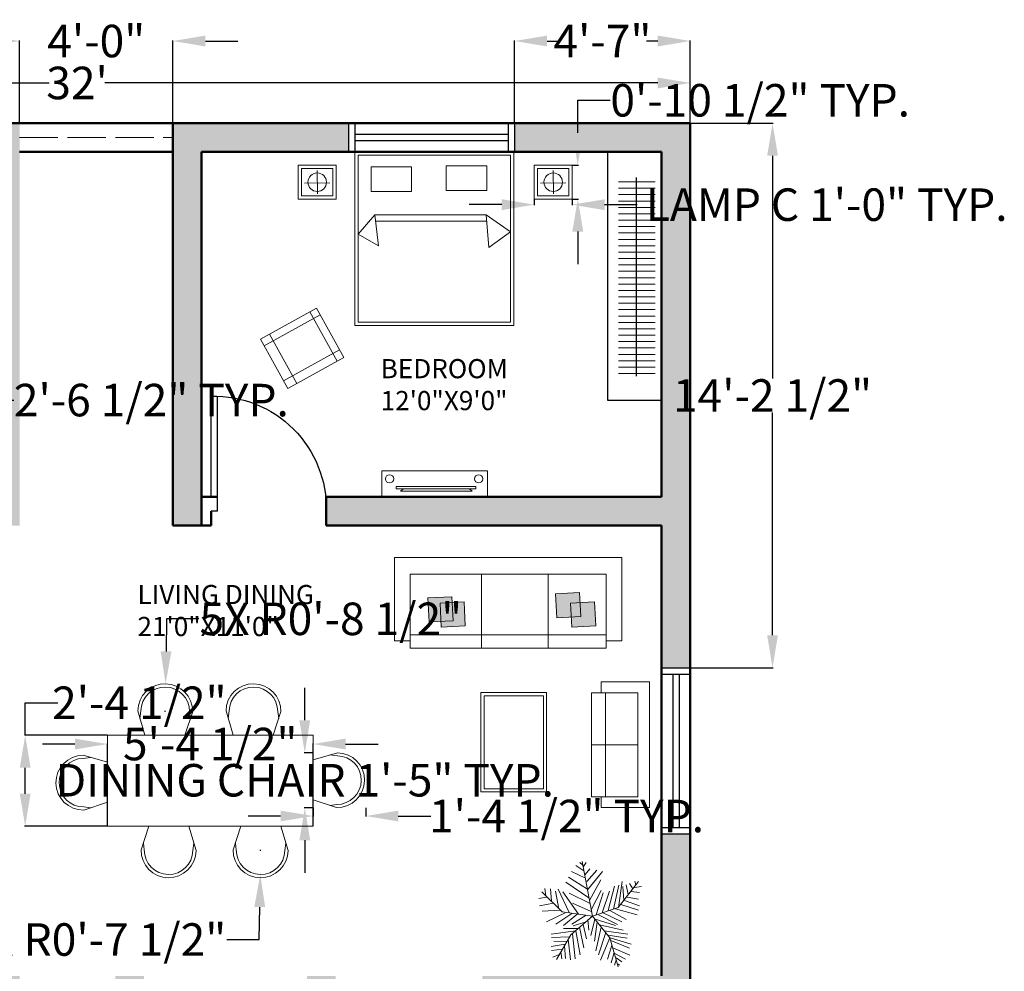
# Model space of a CAD drawing. Units: inches. Extents: x 18 to 9768, y 4 to 3529.
# Tile 6 of 6: x 9424 to 9733, y 3225 to 3523. Entities that reach past the tile are written whole.
import ezdxf

# ---------------------------------------------------------------- set-up
doc = ezdxf.new("R2010")
doc.units = ezdxf.units.IN
doc.header["$MEASUREMENT"] = 0
doc.linetypes.add('ACAD_ISO02W100', pattern=[15, 12, -3])
for name, color, linetype, lineweight in [('A-ANNO-DIMS', 2, 'Continuous', 18), ('A-AREA-IDEN', 7, 'Continuous', 18), ('A-CASE-PATT', 9, 'Continuous', 13), ('A-EQPM', 8, 'Continuous', 18), ('A-FLOR-CASE', 9, 'Continuous', 25), ('A-FURN', 8, 'Continuous', 18), ('A-FURN-PATT', 9, 'Continuous', 13), ('A-WALL-OVHD', 8, 'ACAD_ISO02W100', 18), ('A-WALL-PATT', 252, 'Continuous', 13), ('L-PLNT', 3, 'Continuous', 18), ('WAL', 7, 'Continuous', 50)]:
    doc.layers.add(name, color=color, linetype=linetype, lineweight=lineweight)
doc.layers.add('A-DOOR', color=30, linetype='Continuous', lineweight=25, true_color=0xf8991e)
doc.layers.add('A-GLAZ', color=177, linetype='Continuous', lineweight=25, true_color=0x293189)
doc.styles.get("Standard").update_dxf_attribs({"font": 'arial.ttf'})
doc.dimstyles.get("Standard").update_dxf_attribs({"dimtxt": 10.18, "dimasz": 10.18, "dimexe": 0.18, "dimexo": 0.0625, "dimgap": 0.09, "dimtad": 0, "dimtih": 1, "dimtoh": 1, "dimdec": 0, "dimzin": 0, "dimdsep": 46, "dimlunit": 3, "dimtxsty": 'Standard', "dimcen": 0.09, "dimadec": 0, "dimazin": 0, "dimtfac": 1, "dimtdec": 0, "dimtofl": 0, "dimtmove": 0, "dimatfit": 3, "dimfxl": 1, "dimtolj": 1, "dimtzin": 0, "dimarcsym": 0})

# ---------------------------------------------------------------- blocks, each defined once
blk = doc.blocks.new('*U6')
for p, q in [((-8.737, 47.138), (-17.069, 52.711)), ((-10.186, 53.64), (-13.084, 55.962)), ((0, 0), (-10.5, 57)), ((-9.099, 51.782), (-6.563, 55.962)), ((-7.288, 39.707), (-21.778, 46.673)), ((-7.65, 43.423), (-2.578, 49.46)), ((-5.839, 35.992), (4.667, 48.067)), ((-5.114, 27.632), (10.463, 46.673)), ((-3.665, 19.273), (-27.574, 35.527)), ((-5.114, 28.097), (-24.676, 40.636)), ((-2.941, 16.486), (8.652, 37.85)), ((16.259, 5.805), (23.142, 31.348)), ((22.055, 7.198), (27.489, 32.277)), ((27, 9), (48, 36)), ((27.127, 9.056), (31.112, 35.992)), ((31.836, 30.883), (32.561, 16.486)), ((35.096, 32.741), (37.27, 22.524)), ((38.719, 34.134), (41.979, 28.561)), ((43.791, 29.954), (51.036, 30.883)), ((44.153, 36.456), (45.239, 32.741)), ((-31.5, 4.5), (-52.5, 25.5)), ((-48.585, 21.131), (-49.309, 29.026)), ((-43.513, 28.561), (-42.427, 15.558)), ((-38.442, 26.239), (-34.819, 7.663)), ((-35.544, 28.097), (-24.314, 3.947)), ((-14.533, 2.09), (-30.834, 25.31)), ((-24.314, 23.917), (-2.941, 13.7)), ((-1.129, 6.734), (9.014, 26.704)), ((3.942, 1.625), (11.187, 24.381)), ((10.101, 3.483), (17.708, 26.239)), ((40.53, 25.775), (48.862, 24.846)), ((-47.498, 19.737), (-55.83, 18.344)), ((-40.615, 13.7), (-55.105, 10.913)), ((-20.691, 13.7), (-1.129, 4.876)), ((29.662, 12.307), (48.137, 6.269)), ((33.285, 16.486), (48.862, 10.913)), ((36.183, 19.737), (48.137, 17.88)), ((-33.37, 6.269), (-52.207, 5.34)), ((-28.299, 3.483), (-47.86, -5.805)), ((-21.416, 3.018), (-38.079, -8.128)), ((0, 0), (-31.5, 4.5)), ((-15.982, 2.09), (-30.11, -9.521)), ((0, 0), (-22.5, -19.5)), ((-6.563, 1.161), (-21.416, -8.128)), ((0, 0), (27, 9)), ((0, 0), (18, -22.5)), ((6.478, 1.625), (26.04, -8.592)), ((11.187, 3.483), (30.749, -5.805)), ((18.07, 5.805), (35.096, -3.483)), ((24.229, 7.663), (46.688, 1.625)), ((-6.563, -5.805), (-19.967, -9.985)), ((-9.461, -8.592), (-6.201, -23.453)), ((-4.752, -3.483), (-3.665, -14.629)), ((2.493, -3.019), (-1.491, -20.202)), ((1.769, -2.555), (24.229, -9.521)), ((5.029, -6.27), (2.131, -25.775)), ((7.565, -9.056), (32.198, -14.629)), ((-17.431, -15.094), (-42.789, -18.809)), ((-22.5, -19.5), (-37.5, -45)), ((-15.257, -12.772), (-30.11, -12.772)), ((-20.691, -18.345), (-17.793, -44.352)), ((-17.069, -15.094), (-12.721, -40.172)), ((-13.446, -11.378), (-8.737, -32.741)), ((9.014, -11.378), (3.58, -35.992)), ((14.085, -16.951), (6.478, -40.172)), ((12.274, -15.094), (36.907, -18.809)), ((16.259, -19.738), (36.183, -22.989)), ((-28.299, -29.026), (-42.789, -31.348)), ((-24.314, -21.596), (-42.427, -22.06)), ((-26.849, -26.24), (-40.253, -25.775)), ((-25.038, -23.918), (-22.865, -45.281)), ((18.07, -22.524), (8.289, -45.745)), ((20.244, -30.419), (15.897, -44.816)), ((18, -22.5), (27, -52.5)), ((18.433, -22.524), (40.53, -29.026)), ((19.157, -25.311), (38.719, -33.206)), ((-30.834, -34.135), (-42.427, -35.528)), ((-34.457, -39.708), (-40.978, -42.494)), ((-32.646, -36.921), (-31.921, -44.352)), ((-29.023, -30.884), (-27.936, -43.887)), ((22.78, -37.85), (19.519, -48.532)), ((21.331, -32.741), (39.081, -40.636)), ((22.78, -38.314), (34.372, -44.816)), ((24.591, -45.745), (23.142, -50.854)), ((24.591, -43.423), (30.749, -47.603)), ((26.764, -49.925), (28.213, -50.854))]:
    blk.add_line(p, q)
blk = doc.blocks.new('*D7')
at = {"layer": 'A-ANNO-DIMS', "color": 0, "lineweight": -2, "transparency": 16777216}
for p, q in [((9250.43, 3490.42), (9250.43, 3503.16)), ((9260.61, 3502.98), (9433.71, 3502.98)), ((9624.25, 3502.98), (9451.16, 3502.98)), ((9634.43, 3490.42), (9634.43, 3503.16))]:
    blk.add_line(p, q, dxfattribs=at)
at = {"layer": 'A-ANNO-DIMS', "color": 0, "transparency": 16777216}
for points in [[(9260.61, 3504.67), (9260.61, 3501.28), (9250.43, 3502.98)], [(9624.25, 3504.67), (9624.25, 3501.28), (9634.43, 3502.98)]]:
    blk.add_solid(points, dxfattribs=at)
at = {"layer": 'Defpoints', "color": 0, "transparency": 16777216}
for p in [(9634.43, 3502.98), (9250.43, 3490.36), (9634.43, 3490.36)]:
    blk.add_point(p, dxfattribs=at)
at = {"layer": 'A-ANNO-DIMS', "color": 0, "transparency": 16777216, "insert": (9442.43, 3502.98), "char_height": 10.18, "attachment_point": 5}
blk.add_mtext("\\A1;32'", dxfattribs=at)
blk = doc.blocks.new('WINDOW-48')
for p, q in [((0, 0), (0, 9)), ((2, 0), (2, 9)), ((50, 0), (50, 9)), ((52, 0), (52, 9)), ((2, 5.5), (50, 5.5)), ((2, 3.5), (50, 3.5))]:
    blk.add_line(p, q)
blk = doc.blocks.new('DOOR-36-W9')
for p, q in [((2, 36.01), (0, 36.01)), ((2, 36.01), (2, 0.01)), ((0, 31.51), (0, 0.01))]:
    blk.add_line(p, q)
blk.add_arc((1, 35.01), 35.01, 268.3634, 1.6366)
blk = doc.blocks.new('CHAIR-DINING')
for p, q in [((0, 7.62), (2.22, 0)), ((1, 7.61), (0.68, 5.29)), ((14.73, 0), (17.19, 7.39)), ((16.19, 7.4), (16.49, 5.29))]:
    blk.add_line(p, q)
for radius in [8.6, 7.6]:
    blk.add_arc((8.59, 7.51), radius, 359.2162, 179.2162)
blk = doc.blocks.new('NIGHTSTAND-LAMP-C')
for p, q in [((5.92, 8.89), (5.98, 1.61)), ((1.92, 5.01), (9.92, 5.04))]:
    blk.add_line(p, q)
for points in [[(0, 10.55), (0, 10.55), (11.83, 10.55), (11.83, 10.55), (11.83, 0), (11.83, 0), (0, 0), (0, 0)], [(1, 9.55), (10.83, 9.55), (10.83, 1), (1, 1)]]:
    blk.add_lwpolyline(points, close=True)
blk.add_circle((5.92, 5.27), 2.89)
blk = doc.blocks.new('*D36')
at = {"layer": 'A-ANNO-DIMS', "color": 0, "lineweight": -2, "transparency": 16777216}
for p, q in [((9382.16, 3399.2), (9382.16, 3403.86)), ((9392.34, 3403.68), (9402.25, 3403.68)), ((9412.43, 3399.2), (9412.43, 3403.86)), ((9412.43, 3403.68), (9422.61, 3403.68))]:
    blk.add_line(p, q, dxfattribs=at)
at = {"layer": 'A-ANNO-DIMS', "color": 0, "transparency": 16777216}
for points in [[(9392.34, 3405.38), (9392.34, 3401.98), (9382.16, 3403.68)], [(9402.25, 3405.38), (9402.25, 3401.98), (9412.43, 3403.68)]]:
    blk.add_solid(points, dxfattribs=at)
at = {"layer": 'Defpoints', "color": 0, "transparency": 16777216}
for p in [(9412.43, 3403.68), (9382.16, 3399.14), (9412.43, 3399.14)]:
    blk.add_point(p, dxfattribs=at)
at = {"layer": 'A-ANNO-DIMS', "color": 0, "transparency": 16777216, "insert": (9465.68, 3403.68), "char_height": 10.18, "attachment_point": 5}
blk.add_mtext('\\A1;2\'-6 1/2" TYP.', dxfattribs=at)
blk = doc.blocks.new('*D37')
at = {"layer": 'A-ANNO-DIMS', "color": 0, "lineweight": -2, "transparency": 16777216}
for p, q in [((9513.73, 3303.43), (9513.73, 3313.61)), ((9516.25, 3293.25), (9513.55, 3293.25)), ((9516.25, 3276.02), (9513.55, 3276.02)), ((9513.73, 3265.84), (9513.73, 3255.66))]:
    blk.add_line(p, q, dxfattribs=at)
at = {"layer": 'A-ANNO-DIMS', "color": 0, "transparency": 16777216}
for points in [[(9512.03, 3303.43), (9515.42, 3303.43), (9513.73, 3293.25)], [(9512.03, 3265.84), (9515.42, 3265.84), (9513.73, 3276.02)]]:
    blk.add_solid(points, dxfattribs=at)
at = {"layer": 'Defpoints', "color": 0, "transparency": 16777216}
for p in [(9516.31, 3293.25), (9513.73, 3276.02), (9516.31, 3276.02)]:
    blk.add_point(p, dxfattribs=at)
at = {"layer": 'A-ANNO-DIMS', "color": 0, "transparency": 16777216, "insert": (9513.73, 3284.63), "char_height": 10.18, "attachment_point": 5}
blk.add_mtext('\\A1;DINING CHAIR 1\'-5" TYP.', dxfattribs=at)
blk = doc.blocks.new('*D38')
at = {"layer": 'A-ANNO-DIMS', "color": 0, "lineweight": -2, "transparency": 16777216}
for p, q in [((9516.31, 3275.95), (9516.31, 3273.25)), ((9532.82, 3275.95), (9532.82, 3273.25)), ((9506.13, 3273.43), (9495.95, 3273.43)), ((9543, 3273.43), (9553.18, 3273.43))]:
    blk.add_line(p, q, dxfattribs=at)
at = {"layer": 'A-ANNO-DIMS', "color": 0, "transparency": 16777216}
for points in [[(9506.13, 3275.13), (9506.13, 3271.74), (9516.31, 3273.43)], [(9543, 3275.13), (9543, 3271.74), (9532.82, 3273.43)]]:
    blk.add_solid(points, dxfattribs=at)
at = {"layer": 'Defpoints', "color": 0, "transparency": 16777216}
for p in [(9516.31, 3276.02), (9532.82, 3276.02), (9532.82, 3273.43)]:
    blk.add_point(p, dxfattribs=at)
at = {"layer": 'A-ANNO-DIMS', "color": 0, "transparency": 16777216, "insert": (9595.68, 3273.43), "char_height": 10.18, "attachment_point": 5}
blk.add_mtext('\\A1;1\'-4 1/2" TYP.', dxfattribs=at)
blk = doc.blocks.new('*D51')
at = {"layer": 'A-ANNO-DIMS', "color": 0, "lineweight": -2, "transparency": 16777216}
for p, q in [((9585.59, 3466.58), (9585.59, 3464.69)), ((9597.43, 3466.58), (9597.43, 3464.69)), ((9575.41, 3464.87), (9565.23, 3464.87)), ((9607.61, 3464.87), (9617.79, 3464.87))]:
    blk.add_line(p, q, dxfattribs=at)
at = {"layer": 'A-ANNO-DIMS', "color": 0, "transparency": 16777216}
for points in [[(9575.41, 3466.56), (9575.41, 3463.17), (9585.59, 3464.87)], [(9607.61, 3466.56), (9607.61, 3463.17), (9597.43, 3464.87)]]:
    blk.add_solid(points, dxfattribs=at)
at = {"layer": 'Defpoints', "color": 0, "transparency": 16777216}
for p in [(9585.59, 3466.64), (9597.43, 3466.64), (9597.43, 3464.87)]:
    blk.add_point(p, dxfattribs=at)
at = {"layer": 'A-ANNO-DIMS', "color": 0, "transparency": 16777216, "insert": (9677.13, 3464.87), "char_height": 10.18, "attachment_point": 5}
blk.add_mtext('\\A1;LAMP C 1\'-0" TYP.', dxfattribs=at)
blk = doc.blocks.new('*D52')
at = {"layer": 'A-ANNO-DIMS', "color": 0, "lineweight": -2, "transparency": 16777216}
for p, q in [((9599.2, 3487.37), (9599.2, 3497.55)), ((9599.2, 3497.55), (9609.38, 3497.55)), ((9597.49, 3477.19), (9599.38, 3477.19)), ((9597.49, 3466.64), (9599.38, 3466.64)), ((9599.2, 3456.46), (9599.2, 3446.28))]:
    blk.add_line(p, q, dxfattribs=at)
at = {"layer": 'A-ANNO-DIMS', "color": 0, "transparency": 16777216}
for points in [[(9597.51, 3487.37), (9600.9, 3487.37), (9599.2, 3477.19)], [(9597.51, 3456.46), (9600.9, 3456.46), (9599.2, 3466.64)]]:
    blk.add_solid(points, dxfattribs=at)
at = {"layer": 'Defpoints', "color": 0, "transparency": 16777216}
for p in [(9597.43, 3477.19), (9599.2, 3477.19), (9597.43, 3466.64)]:
    blk.add_point(p, dxfattribs=at)
at = {"layer": 'A-ANNO-DIMS', "color": 0, "transparency": 16777216, "insert": (9656.31, 3497.55), "char_height": 10.18, "attachment_point": 5}
blk.add_mtext('\\A1;0\'-10 1/2" TYP.', dxfattribs=at)
blk = doc.blocks.new('*D72')
at = {"layer": 'A-ANNO-DIMS', "color": 0, "lineweight": -2, "transparency": 16777216}
for p, q in [((9414.25, 3516.11), (9404.07, 3516.11)), ((9424.43, 3490.42), (9424.43, 3516.29)), ((9472.43, 3490.42), (9472.43, 3516.29)), ((9482.61, 3516.11), (9492.79, 3516.11))]:
    blk.add_line(p, q, dxfattribs=at)
at = {"layer": 'A-ANNO-DIMS', "color": 0, "transparency": 16777216}
for points in [[(9414.25, 3517.81), (9414.25, 3514.41), (9424.43, 3516.11)], [(9482.61, 3517.81), (9482.61, 3514.41), (9472.43, 3516.11)]]:
    blk.add_solid(points, dxfattribs=at)
at = {"layer": 'Defpoints', "color": 0, "transparency": 16777216}
for p in [(9472.43, 3516.11), (9424.43, 3490.36), (9472.43, 3490.36)]:
    blk.add_point(p, dxfattribs=at)
at = {"layer": 'A-ANNO-DIMS', "color": 0, "transparency": 16777216, "insert": (9448.43, 3516.11), "char_height": 10.18, "attachment_point": 5}
blk.add_mtext('\\A1;4\'-0"', dxfattribs=at)
blk = doc.blocks.new('*D74')
at = {"layer": 'A-ANNO-DIMS', "color": 0, "lineweight": -2, "transparency": 16777216}
for p, q in [((9579.43, 3490.42), (9579.43, 3516.29)), ((9589.61, 3516.11), (9593.11, 3516.11)), ((9624.25, 3516.11), (9620.76, 3516.11)), ((9634.43, 3490.42), (9634.43, 3516.29))]:
    blk.add_line(p, q, dxfattribs=at)
at = {"layer": 'A-ANNO-DIMS', "color": 0, "transparency": 16777216}
for points in [[(9589.61, 3517.81), (9589.61, 3514.41), (9579.43, 3516.11)], [(9624.25, 3517.81), (9624.25, 3514.41), (9634.43, 3516.11)]]:
    blk.add_solid(points, dxfattribs=at)
at = {"layer": 'Defpoints', "color": 0, "transparency": 16777216}
for p in [(9634.43, 3516.11), (9579.43, 3490.36), (9634.43, 3490.36)]:
    blk.add_point(p, dxfattribs=at)
at = {"layer": 'A-ANNO-DIMS', "color": 0, "transparency": 16777216, "insert": (9606.93, 3516.11), "char_height": 10.18, "attachment_point": 5}
blk.add_mtext('\\A1;4\'-7"', dxfattribs=at)
blk = doc.blocks.new('*D77')
at = {"layer": 'A-ANNO-DIMS', "color": 0, "lineweight": -2, "transparency": 16777216}
for p, q in [((9634.5, 3490.36), (9660.36, 3490.36)), ((9660.18, 3480.18), (9660.18, 3410.46)), ((9660.18, 3330.04), (9660.18, 3399.76)), ((9634.5, 3319.86), (9660.36, 3319.86))]:
    blk.add_line(p, q, dxfattribs=at)
at = {"layer": 'A-ANNO-DIMS', "color": 0, "transparency": 16777216}
for points in [[(9658.49, 3480.18), (9661.88, 3480.18), (9660.18, 3490.36)], [(9658.49, 3330.04), (9661.88, 3330.04), (9660.18, 3319.86)]]:
    blk.add_solid(points, dxfattribs=at)
at = {"layer": 'Defpoints', "color": 0, "transparency": 16777216}
for p in [(9634.43, 3490.36), (9660.18, 3490.36), (9634.43, 3319.86)]:
    blk.add_point(p, dxfattribs=at)
at = {"layer": 'A-ANNO-DIMS', "color": 0, "transparency": 16777216, "insert": (9660.18, 3405.11), "char_height": 10.18, "attachment_point": 5}
blk.add_mtext('\\A1;14\'-2 1/2"', dxfattribs=at)
blk = doc.blocks.new('*D79')
at = {"layer": 'A-ANNO-DIMS', "color": 0, "lineweight": -2, "transparency": 16777216}
for p, q in [((9441.75, 3295.97), (9431.57, 3295.97)), ((9451.93, 3270.28), (9451.93, 3296.15)), ((9516.31, 3270.28), (9516.31, 3296.15)), ((9526.49, 3295.97), (9536.67, 3295.97))]:
    blk.add_line(p, q, dxfattribs=at)
at = {"layer": 'A-ANNO-DIMS', "color": 0, "transparency": 16777216}
for points in [[(9441.75, 3297.66), (9441.75, 3294.27), (9451.93, 3295.97)], [(9526.49, 3297.66), (9526.49, 3294.27), (9516.31, 3295.97)]]:
    blk.add_solid(points, dxfattribs=at)
at = {"layer": 'Defpoints', "color": 0, "transparency": 16777216}
for p in [(9516.31, 3295.97), (9451.93, 3270.22), (9516.31, 3270.22)]:
    blk.add_point(p, dxfattribs=at)
at = {"layer": 'A-ANNO-DIMS', "color": 0, "transparency": 16777216, "insert": (9484.12, 3295.97), "char_height": 10.18, "attachment_point": 5}
blk.add_mtext('\\A1;5\'-4 1/2"', dxfattribs=at)
blk = doc.blocks.new('*D80')
at = {"layer": 'A-ANNO-DIMS', "color": 0, "lineweight": -2, "transparency": 16777216}
for p, q in [((9426.18, 3298.72), (9426.18, 3308.9)), ((9426.18, 3308.9), (9436.36, 3308.9)), ((9451.87, 3298.72), (9426, 3298.72)), ((9426.18, 3280.4), (9426.18, 3288.54)), ((9451.87, 3270.22), (9426, 3270.22))]:
    blk.add_line(p, q, dxfattribs=at)
at = {"layer": 'A-ANNO-DIMS', "color": 0, "transparency": 16777216}
for points in [[(9424.48, 3288.54), (9427.88, 3288.54), (9426.18, 3298.72)], [(9424.48, 3280.4), (9427.88, 3280.4), (9426.18, 3270.22)]]:
    blk.add_solid(points, dxfattribs=at)
at = {"layer": 'Defpoints', "color": 0, "transparency": 16777216}
for p in [(9426.18, 3298.72), (9451.93, 3298.72), (9451.93, 3270.22)]:
    blk.add_point(p, dxfattribs=at)
at = {"layer": 'A-ANNO-DIMS', "color": 0, "transparency": 16777216, "insert": (9461.93, 3308.9), "char_height": 10.18, "attachment_point": 5}
blk.add_mtext('\\A1;2\'-4 1/2"', dxfattribs=at)
blk = doc.blocks.new('*D83')
at = {"layer": 'A-ANNO-DIMS', "color": 0, "lineweight": -2, "transparency": 16777216}
for p, q in [((9470.42, 3335.18), (9470.28, 3325)), ((9480.6, 3335.18), (9470.42, 3335.18)), ((9469.93, 3306.23), (9470.11, 3306.23)), ((9470.02, 3306.14), (9470.02, 3306.32))]:
    blk.add_line(p, q, dxfattribs=at)
at = {"layer": 'A-ANNO-DIMS', "color": 0, "transparency": 16777216}
blk.add_solid([(9468.58, 3325.03), (9471.97, 3324.98), (9470.14, 3314.82)], dxfattribs=at)
at = {"layer": 'Defpoints', "color": 0, "transparency": 16777216}
for p in [(9470.14, 3314.82), (9470.02, 3306.23)]:
    blk.add_point(p, dxfattribs=at)
at = {"layer": 'A-ANNO-DIMS', "color": 0, "transparency": 16777216, "insert": (9521.89, 3335.18), "char_height": 10.18, "attachment_point": 5}
blk.add_mtext('\\A1;5X R0\'-8 1/2"', dxfattribs=at)
blk = doc.blocks.new('*D84')
at = {"layer": 'A-ANNO-DIMS', "color": 0, "lineweight": -2, "transparency": 16777216}
for p, q in [((9499.78, 3262.71), (9499.96, 3262.71)), ((9499.87, 3262.62), (9499.87, 3262.8)), ((9499.49, 3234.76), (9499.63, 3244.93)), ((9489.31, 3234.76), (9499.49, 3234.76))]:
    blk.add_line(p, q, dxfattribs=at)
at = {"layer": 'A-ANNO-DIMS', "color": 0, "transparency": 16777216}
blk.add_solid([(9497.93, 3244.96), (9501.32, 3244.91), (9499.77, 3255.11)], dxfattribs=at)
at = {"layer": 'Defpoints', "color": 0, "transparency": 16777216}
for p in [(9499.87, 3262.71), (9499.77, 3255.11)]:
    blk.add_point(p, dxfattribs=at)
at = {"layer": 'A-ANNO-DIMS', "color": 0, "transparency": 16777216, "insert": (9448.02, 3234.76), "char_height": 10.18, "attachment_point": 5}
blk.add_mtext('\\A1;5X R0\'-7 1/2"', dxfattribs=at)

msp = doc.modelspace()

# ---------------------------------------------------------------- hatches: boundary and pattern name
at = {"layer": 'A-CASE-PATT'}
h = msp.add_hatch(dxfattribs=at)
h.set_pattern_fill('ANSI31', color=256, scale=16, angle=-45, style=0)
h.paths.add_polyline_path([(9612, 3410.74), (9623.39, 3410.74), (9623.39, 3472.74), (9612, 3472.74)])
at = {"layer": 'A-FURN-PATT'}
h = msp.add_hatch(color=256, dxfattribs=at)
h.dxf.hatch_style = 1
h.paths.add_polyline_path([(9560.14, 3334.56), (9559.78, 3342.08), (9552.26, 3341.72), (9552.62, 3334.2)])
h = msp.add_hatch(color=256, dxfattribs=at)
h.dxf.hatch_style = 1
h.paths.add_polyline_path([(9600.12, 3335.86), (9599.76, 3343.38), (9592.24, 3343.02), (9592.61, 3335.5)])
h = msp.add_hatch(color=256, dxfattribs=at)
h.dxf.hatch_style = 1
h.paths.add_polyline_path([(9563.99, 3332.96), (9563.62, 3340.48), (9556.11, 3340.12), (9556.47, 3332.6)])
h = msp.add_hatch(color=256, dxfattribs=at)
h.dxf.hatch_style = 1
h.paths.add_polyline_path([(9604.82, 3332.96), (9604.46, 3340.48), (9596.94, 3340.11), (9597.31, 3332.59)])
at = {"layer": 'A-WALL-PATT'}
h = msp.add_hatch(color=256, dxfattribs=at)
h.dxf.hatch_style = 1
h.paths.add_polyline_path([(9424.43, 3490.36), (9363.42, 3490.36), (9363.42, 3481.36), (9373.43, 3481.36), (9382.43, 3481.36), (9415.43, 3481.36), (9415.43, 3373.36), (9415.43, 3364.36), (9424.43, 3364.36), (9424.43, 3373.36), (9424.43, 3481.36)])
h.paths.add_polyline_path([(9527.43, 3490.36), (9472.43, 3490.36), (9472.43, 3481.36), (9472.43, 3373.36), (9472.43, 3364.36), (9481.43, 3364.36), (9481.43, 3373.36), (9481.43, 3481.36), (9527.43, 3481.36)])
h.paths.add_polyline_path([(9311.42, 3490.36), (9250.43, 3490.36), (9250.43, 3353.86), (9259.43, 3353.86), (9259.43, 3364.36), (9301.43, 3364.36), (9301.43, 3315.36), (9301.43, 3306.36), (9310.43, 3306.36), (9310.43, 3315.36), (9310.43, 3364.36), (9382.43, 3364.36), (9382.43, 3368.86, -0.017236), (9382.43, 3370.86), (9382.43, 3373.36), (9259.43, 3373.36), (9259.43, 3481.36), (9311.42, 3481.36)])
h.paths.add_polyline_path([(9376.43, 3216.86, -0.014283), (9376.43, 3218.86), (9376.43, 3223.36), (9259.43, 3223.36), (9259.43, 3238.86), (9250.43, 3238.86), (9250.43, 3058.36), (9311.43, 3058.36), (9311.43, 3067.36), (9259.43, 3067.36), (9259.43, 3214.36), (9376.43, 3214.36)])
h.paths.add_polyline_path([(9382.43, 3364.36), (9373.43, 3364.36), (9373.43, 3315.36), (9347, 3315.36), (9347, 3306.36), (9382.43, 3306.36)], flags=0)
h.paths.add_polyline_path([(9277.41, 3315.36), (9259.43, 3315.36), (9259.43, 3325.86), (9250.43, 3325.86), (9250.43, 3290.86), (9259.43, 3290.86), (9259.43, 3306.36), (9277.41, 3306.36)])
h.paths.add_polyline_path([(9424.43, 3214.36), (9424.43, 3223.36), (9415.43, 3223.36), (9415.43, 3214.36), (9415.43, 3106.36), (9417.93, 3106.36, -0.014283), (9419.93, 3106.36), (9424.43, 3106.36), (9424.43, 3109.36), (9424.43, 3118.36)])
h.paths.add_polyline_path([(9463.43, 3214.36), (9463.43, 3223.36), (9454.43, 3223.36), (9454.43, 3214.36), (9454.43, 3118.36), (9454.43, 3109.36), (9548.43, 3109.36), (9548.43, 3118.36), (9523.43, 3118.36), (9523.43, 3144.21), (9518.93, 3144.21, -0.017236), (9516.93, 3144.21), (9514.43, 3144.21), (9514.43, 3118.36), (9463.43, 3118.36)])
h.paths.add_polyline_path([(9523.43, 3214.36), (9523.43, 3223.36), (9514.43, 3223.36), (9514.43, 3214.36), (9514.43, 3177.21), (9523.43, 3177.21)], flags=17)
h.paths.add_polyline_path([(9514.43, 3193.54), (9463.43, 3193.54), (9463.43, 3184.54), (9514.43, 3184.54)], flags=17)
h.paths.add_polyline_path([(9634.43, 3267.86), (9625.43, 3267.86), (9625.43, 3223.36), (9569.35, 3223.36), (9569.35, 3214.36), (9625.43, 3214.36), (9625.43, 3118.36), (9600.43, 3118.36), (9600.43, 3109.36), (9625.43, 3109.36), (9634.43, 3109.36)])
h.paths.add_polyline_path([(9634.43, 3490.36), (9579.43, 3490.36), (9579.43, 3481.36), (9625.43, 3481.36), (9625.43, 3373.36), (9520.43, 3373.36), (9520.43, 3370.86, -0.014283), (9520.43, 3368.86), (9520.43, 3364.36), (9625.43, 3364.36), (9625.43, 3319.86), (9634.43, 3319.86)])
h.paths.add_polyline_path([(9424.43, 3067.36), (9415.43, 3067.36), (9363.43, 3067.36), (9363.43, 3058.36), (9424.43, 3058.36)])

# ---------------------------------------------------------------- linework, layer by layer
at = {"layer": 'A-EQPM'}
for p, q in [((9544.59, 3375.86), (9543.74, 3375.11)), ((9566.17, 3375.11), (9565.34, 3375.86)), ((9543.74, 3375.11), (9566.17, 3375.11))]:
    msp.add_line(p, q, dxfattribs=at)
for points in [[(9537.86, 3373.36), (9537.86, 3373.36), (9570.9, 3373.36), (9570.9, 3373.36), (9570.9, 3381.56), (9570.9, 3381.56), (9537.86, 3381.56), (9537.86, 3381.56)], [(9542.38, 3376.58), (9542.38, 3376.58), (9567.27, 3376.58), (9567.27, 3376.58), (9567.27, 3375.86), (9567.27, 3375.86), (9542.38, 3375.86), (9542.38, 3375.86)]]:
    msp.add_lwpolyline(points, close=True, dxfattribs=at)
for centre in [(9540.27, 3379.02), (9568.16, 3379.02)]:
    msp.add_circle(centre, 1.29, dxfattribs=at)
at = {"layer": 'A-FLOR-CASE'}
for p, q in [((9608.53, 3481.36), (9608.53, 3403.69)), ((9617.51, 3473.39), (9617.51, 3411.2)), ((9608.53, 3403.69), (9625.43, 3403.69))]:
    msp.add_line(p, q, dxfattribs=at)
at = {"layer": 'A-FURN'}
for p, q in [((9535.62, 3461.65), (9530.43, 3455.66)), ((9535.62, 3461.65), (9570.5, 3461.65)), ((9536.85, 3451.96), (9535.62, 3461.65)), ((9535.87, 3459.68), (9570.67, 3459.74)), ((9570.5, 3461.65), (9578.16, 3456.4)), ((9571.38, 3451.47), (9570.5, 3461.65)), ((9578.16, 3456.4), (9571.38, 3451.47)), ((9530.43, 3455.66), (9536.85, 3451.96)), ((9515.33, 3431.35), (9523.9, 3415.91)), ((9500.96, 3420.68), (9518.52, 3430.42)), ((9502.66, 3424.32), (9511.22, 3408.88)), ((9507.06, 3409.69), (9524.62, 3419.43)), ((9569.03, 3349.18), (9569.03, 3326)), ((9589.97, 3349.18), (9589.97, 3326)), ((9546.67, 3330.14), (9608.09, 3330.14)), ((9607.85, 3312.05), (9607.85, 3279.42)), ((9463.64, 3298.72), (9476.16, 3298.72)), ((9617.98, 3295.73), (9603.52, 3295.73))]:
    msp.add_line(p, q, dxfattribs=at)
for points in [[(9529.43, 3481.36), (9529.43, 3481.36), (9579.16, 3481.36), (9579.16, 3481.36), (9579.16, 3427.04), (9579.16, 3427.04), (9529.43, 3427.04), (9529.43, 3427.04)], [(9530.43, 3480.36), (9578.16, 3480.36), (9578.16, 3428.04), (9530.43, 3428.04)], [(9534.5, 3476.73), (9534.5, 3476.73), (9547.14, 3476.73), (9547.14, 3476.73), (9547.14, 3468.97), (9547.14, 3468.97), (9534.5, 3468.97), (9534.5, 3468.97)], [(9558.04, 3477.06), (9558.04, 3477.06), (9570.68, 3477.06), (9570.68, 3477.06), (9570.68, 3469.29), (9570.68, 3469.29), (9558.04, 3469.29), (9558.04, 3469.29)], [(9499.81, 3422.74), (9499.81, 3422.74), (9517.37, 3432.49), (9517.37, 3432.49), (9525.94, 3417.04), (9525.94, 3417.04), (9508.38, 3407.3), (9508.38, 3407.3)], [(9608.09, 3349.18), (9608.09, 3349.18), (9546.67, 3349.18), (9546.67, 3349.18), (9546.67, 3326), (9546.67, 3326), (9608.09, 3326), (9608.09, 3326)], [(9552.26, 3341.72), (9552.62, 3334.2), (9560.14, 3334.56), (9559.78, 3342.08)], [(9592.24, 3343.02), (9592.61, 3335.5), (9600.12, 3335.86), (9599.76, 3343.38)], [(9556.11, 3340.12), (9556.47, 3332.6), (9563.99, 3332.96), (9563.62, 3340.48)], [(9596.94, 3340.11), (9597.31, 3332.59), (9604.82, 3332.96), (9604.46, 3340.48)], [(9568.89, 3312.1), (9568.89, 3312.1), (9589.44, 3312.1), (9589.44, 3312.1), (9589.44, 3280.99), (9589.44, 3280.99), (9568.89, 3280.99), (9568.89, 3280.99)], [(9569.89, 3311.1), (9588.44, 3311.1), (9588.44, 3281.99), (9569.89, 3281.99)], [(9617.98, 3312.05), (9617.98, 3312.05), (9603.52, 3312.05), (9603.52, 3312.05), (9603.52, 3279.42), (9603.52, 3279.42), (9617.98, 3279.42), (9617.98, 3279.42)], [(9451.93, 3298.72), (9451.93, 3298.72), (9516.31, 3298.72), (9516.31, 3298.72), (9516.31, 3270.22), (9516.31, 3270.22), (9451.93, 3270.22), (9451.93, 3270.22)]]:
    msp.add_lwpolyline(points, close=True, dxfattribs=at)
for points in [[(9546.67, 3354.37), (9546.67, 3354.37), (9541.77, 3354.37), (9541.77, 3354.37), (9541.77, 3328.26), (9541.77, 3328.26), (9546.67, 3328.26), (9546.67, 3328.26), (9546.67, 3349.18)], [(9608.09, 3354.37), (9608.09, 3354.37), (9546.67, 3354.37), (9546.67, 3354.37)], [(9608.09, 3349.18), (9608.09, 3328.26), (9608.09, 3328.26), (9612.98, 3328.26), (9612.98, 3328.26), (9612.98, 3354.37), (9612.98, 3354.37), (9608.09, 3354.37), (9608.09, 3354.37)], [(9546.67, 3349.18), (9546.67, 3349.18), (9608.09, 3349.18), (9608.09, 3349.18)], [(9617.98, 3312.05), (9606.57, 3312.05), (9606.57, 3312.05), (9606.57, 3315.4), (9606.57, 3315.4), (9621.69, 3315.4), (9621.69, 3315.4), (9621.69, 3312.05)], [(9617.98, 3279.41), (9617.98, 3279.41), (9617.98, 3312.05)], [(9621.69, 3312.05), (9621.69, 3312.05), (9621.69, 3279.41), (9621.69, 3279.41)], [(9621.69, 3279.42), (9621.69, 3279.42), (9621.69, 3276.07), (9621.69, 3276.07), (9606.57, 3276.07), (9606.57, 3276.07), (9606.57, 3279.42), (9606.57, 3279.42), (9617.98, 3279.42)]]:
    msp.add_lwpolyline(points, dxfattribs=at)
at = {"layer": 'A-WALL-OVHD'}
msp.add_line((9424.43, 3485.86), (9472.43, 3485.86), dxfattribs=at)
at = {"layer": 'WAL'}
for p, q in [((9250.43, 3490.36), (9634.43, 3490.36)), ((9472.43, 3481.36), (9472.43, 3490.36)), ((9634.43, 3490.36), (9634.43, 3058.36)), ((9424.43, 3481.36), (9472.43, 3481.36)), ((9472.43, 3481.36), (9472.43, 3373.36)), ((9481.43, 3481.36), (9481.43, 3373.36)), ((9481.43, 3481.36), (9625.43, 3481.36)), ((9625.43, 3481.36), (9625.43, 3373.36)), ((9472.43, 3373.36), (9472.43, 3364.36)), ((9481.43, 3373.36), (9486.43, 3373.36)), ((9481.43, 3373.36), (9481.43, 3364.36)), ((9520.27, 3373.36), (9625.43, 3373.36)), ((9520.43, 3373.36), (9520.43, 3364.36)), ((9484.43, 3368.86), (9484.43, 3364.36)), ((9472.43, 3364.36), (9484.43, 3364.36)), ((9520.43, 3364.36), (9625.43, 3364.36)), ((9625.43, 3364.36), (9625.43, 3223.36))]:
    msp.add_line(p, q, dxfattribs=at)

# ---------------------------------------------------------------- block references
at = {"layer": 'A-DOOR', "extrusion": (0, 0, -1), "zscale": -1, "rotation": 180}
msp.add_blockref('DOOR-36-W9', (-9484.43, 3404.87), dxfattribs=at)
at = {"layer": 'A-FURN'}
for name, p in [('NIGHTSTAND-LAMP-C', (9511.69, 3466.64)), ('NIGHTSTAND-LAMP-C', (9585.59, 3466.64)), ('CHAIR-DINING', (9461.43, 3298.72)), ('CHAIR-DINING', (9489.07, 3298.72))]:
    msp.add_blockref(name, p, dxfattribs=at)
for p, rotation in [((9516.31, 3293.25), 270.0000000000082), ((9479.67, 3270.22), 180), ((9508.47, 3270.22), 180)]:
    msp.add_blockref('CHAIR-DINING', p, dxfattribs=dict(at, rotation=rotation))
at = {"layer": 'A-FURN', "extrusion": (0, 0, -1), "zscale": -1, "rotation": 270.0000000000076}
msp.add_blockref('CHAIR-DINING', (-9451.93, 3292.47), dxfattribs=at)
at = {"layer": 'A-GLAZ'}
for p, rotation in [((9579.43, 3490.36), 180), ((9625.43, 3319.86), 269.999999999992)]:
    msp.add_blockref('WINDOW-48', p, dxfattribs=dict(at, rotation=rotation))
at = {"layer": 'L-PLNT', "xscale": 0.300939006580229, "yscale": 0.300939006580229, "zscale": 0.300939006580229}
msp.add_blockref('*U6', (9603.77, 3242.05), dxfattribs=at)

# ---------------------------------------------------------------- texts
at = {"layer": 'A-AREA-IDEN', "char_height": 6, "attachment_point": 1}
for s, insert in [('BEDROOM\\P12\'0"X9\'0"', (9537.48, 3416.52)), ('LIVING DINING\\P21\'0"X11\'0"', (9461.34, 3345.78))]:
    msp.add_mtext_dynamic_manual_height_columns(s, width=61.6465, gutter_width=1, heights=[0], dxfattribs=dict(at, insert=insert))

# ---------------------------------------------------------------- dimensions: what is measured, and where the dimension line sits
at = {"layer": 'A-ANNO-DIMS'}
for base, p1, p2, override, picture, middle in [((9472.43, 3516.11), (9424.43, 3490.36), (9472.43, 3490.36), {"dimdec": 1, "dimlfac": 1, "dimrnd": 0, "dimzin": 1, "dimdsep": 46, "dimlunit": 4, "dimfrac": 2}, '*D72', (9448.43, 3516.11)), ((9634.43, 3516.11), (9579.43, 3490.36), (9634.43, 3490.36), {"dimdec": 1, "dimlfac": 1, "dimrnd": 0, "dimzin": 1, "dimdsep": 46, "dimlunit": 4, "dimfrac": 2}, '*D74', (9606.93, 3516.11)), ((9634.43, 3502.98), (9250.43, 3490.36), (9634.43, 3490.36), {"dimclrd": 0, "dimclre": 0, "dimclrt": 0}, '*D7', (9442.43, 3502.98)), ((9516.31, 3295.97), (9451.93, 3270.22), (9516.31, 3270.22), {"dimdec": 1, "dimlfac": 1, "dimrnd": 0, "dimzin": 1, "dimdsep": 46, "dimlunit": 4, "dimfrac": 2}, '*D79', (9484.12, 3295.97))]:
    dim = msp.add_linear_dim(base=base, p1=p1, p2=p2, dimstyle='Standard', override=override, dxfattribs=at)
    dim.commit()
    dim.dimension.update_dxf_attribs({"geometry": picture, "text_midpoint": middle})
for base, p1, p2, angle, text, picture, middle in [((9599.2019, 3477.1873), (9597.4269, 3466.6412), (9597.4269, 3477.1873), 90, '<> TYP.', '*D52', (9656.3131, 3497.5473)), ((9513.73, 3276.02), (9516.31, 3293.25), (9516.31, 3276.02), 270, 'DINING CHAIR <> TYP.', '*D37', (9513.73, 3284.63)), ((9532.82, 3273.43), (9516.31, 3276.02), (9532.82, 3276.02), 0, '<> TYP.', '*D38', (9595.68, 3273.43))]:
    dim = msp.add_linear_dim(base=base, p1=p1, p2=p2, angle=angle, text=text, dimstyle='Standard', override={"dimdec": 1, "dimlfac": 1, "dimrnd": 0, "dimzin": 1, "dimdsep": 46, "dimlunit": 4, "dimfrac": 2}, dxfattribs=at)
    dim.commit()
    dim.dimension.update_dxf_attribs({"geometry": picture, "text_midpoint": middle})
for base, p1, p2, text, picture, middle in [((9597.43, 3464.87), (9585.59, 3466.64), (9597.43, 3466.64), 'LAMP C <> TYP.', '*D51', (9677.13, 3464.87)), ((9412.43, 3403.68), (9382.16, 3399.14), (9412.43, 3399.14), '<> TYP.', '*D36', (9465.68, 3403.68))]:
    dim = msp.add_linear_dim(base=base, p1=p1, p2=p2, text=text, dimstyle='Standard', override={"dimdec": 1, "dimlfac": 1, "dimrnd": 0, "dimzin": 1, "dimdsep": 46, "dimlunit": 4, "dimfrac": 2}, dxfattribs=at)
    dim.commit()
    dim.dimension.update_dxf_attribs({"geometry": picture, "text_midpoint": middle})
for base, p1, p2, picture, middle in [((9660.18, 3490.36), (9634.43, 3319.86), (9634.43, 3490.36), '*D77', (9660.18, 3405.11)), ((9426.18, 3298.72), (9451.93, 3270.22), (9451.93, 3298.72), '*D80', (9461.93, 3308.9))]:
    dim = msp.add_linear_dim(base=base, p1=p1, p2=p2, angle=90, dimstyle='Standard', override={"dimdec": 1, "dimlfac": 1, "dimrnd": 0, "dimzin": 1, "dimdsep": 46, "dimlunit": 4, "dimfrac": 2}, dxfattribs=at)
    dim.commit()
    dim.dimension.update_dxf_attribs({"geometry": picture, "text_midpoint": middle})
for center, mpoint, picture, middle in [((9470.02, 3306.23), (9470.14, 3314.82), '*D83', (9521.89, 3335.18)), ((9499.87, 3262.71), (9499.77, 3255.11), '*D84', (9448.02, 3234.76))]:
    dim = msp.add_radius_dim(center=center, mpoint=mpoint, text='5X <>', dimstyle='Standard', override={"dimdec": 1, "dimlfac": 1, "dimrnd": 0, "dimzin": 1, "dimdsep": 46, "dimlunit": 4, "dimfrac": 2}, dxfattribs=at)
    dim.commit()
    dim.dimension.update_dxf_attribs({"geometry": picture, "text_midpoint": middle})

doc.saveas('drawing.dxf')
